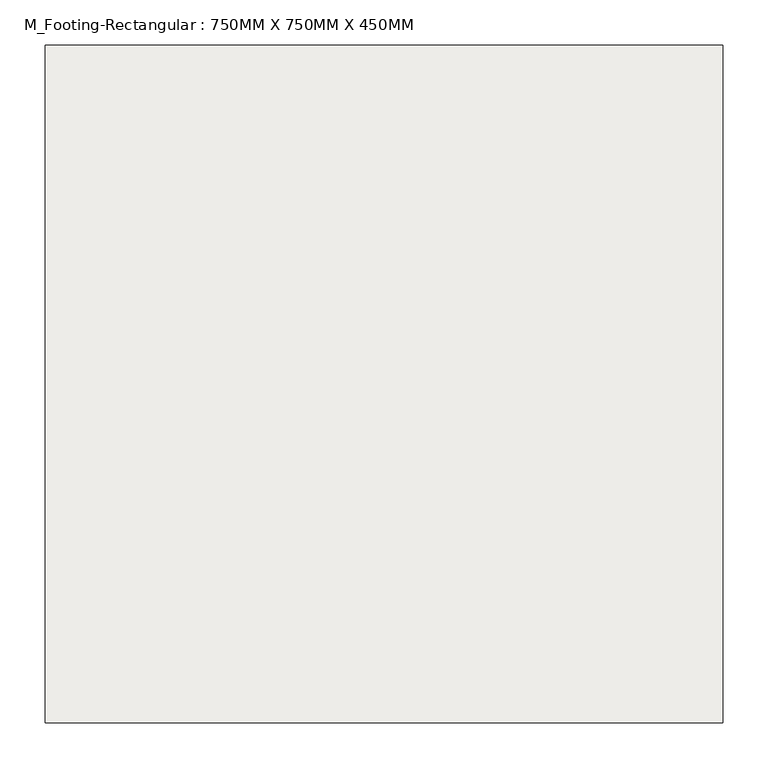
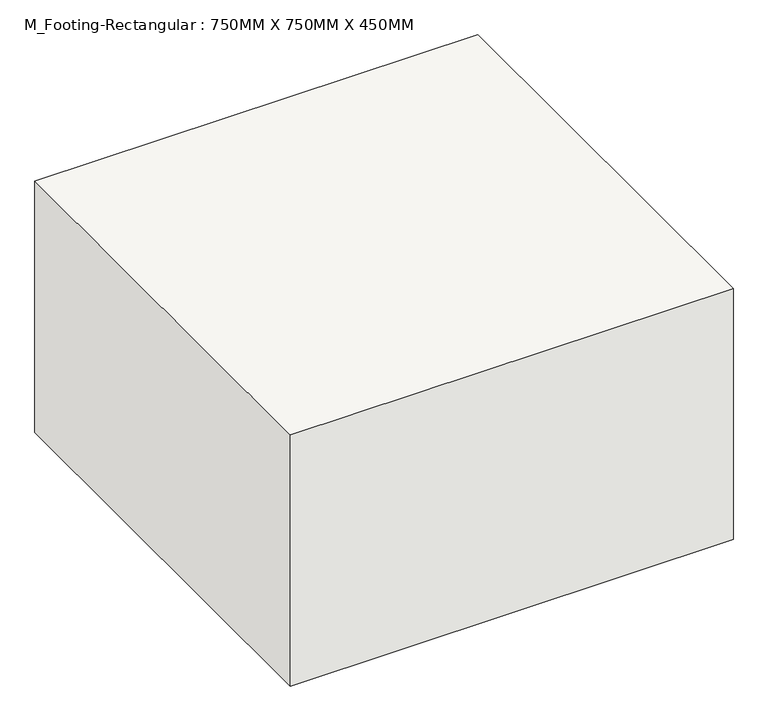
"""IFC4 building model written with IfcOpenShell, lengths in millimetres: slab geometry, M_Footing-Rectangular : 750MM X 750MM X 450MM."""

from ifc_helpers import new_model, si_unit, frame, origin, place, context, project, spatial, polyline, outline, extrude, source, transform, mapped, element, save


def m_footing_rectangular_750mm_x_750mm_x_450mm_d1bf6791(model_context):
    return source(origin(), model_context, "Body", "SweptSolid", [
        extrude(outline(polyline([(375.0, 375.0), (375.0, -375.0), (-375.0, -375.0), (-375.0, 375.0), (375.0, 375.0)])), frame((0.0, 0.0, -450.0), z_axis=(0.0, 0.0, 1.0), x_axis=(1.0, 0.0, 0.0)), (0.0, 0.0, 1.0), 450.0),
    ])


if __name__ == "__main__":
    model = new_model("IFC4")
    model_context = context("Model", 3, world=origin())
    ifc_project = project(units=[si_unit("LENGTHUNIT", "METRE", prefix="MILLI")], contexts=[model_context])
    site = spatial("IfcSite", under=ifc_project)
    building = spatial("IfcBuilding", under=site)
    placement = place(None, origin())
    m_footing_rectangular_750mm_x_750mm_x_450mm_shape = m_footing_rectangular_750mm_x_750mm_x_450mm_d1bf6791(model_context)
    element("IfcSlab", 1, ObjectType="M_Footing-Rectangular : 750MM X 750MM X 450MM", at=placement, inside=building, context=model_context, shape_type="MappedRepresentation", body=[
        mapped(m_footing_rectangular_750mm_x_750mm_x_450mm_shape, transform((0.0, 0.0, 0.0), x_axis=(1.0, 0.0, 0.0), y_axis=(0.0, 1.0, 0.0), z_axis=(0.0, 0.0, 1.0))),
    ])
    save(model, "model.ifc")

# Revit data of these elements
# Type "M_Footing-Rectangular : 750MM X 750MM X 450MM"
#   Width = 750 mm
#   Length = 750 mm
#   Foundation Thickness = 450 mm
#   Structural Material [instance default] = Concrete, Cast-in-Place gray
#   Assembly Code = ""
# Element 1 (IfcSlab, "M_Footing-Rectangular : 750MM X 750MM X 450MM")
#   Materials on its faces: "Concrete, Cast-in-Place gray"
# Materials
#   "Concrete, Cast-in-Place gray": class "Concrete", colour RGB 192 192 192, transparency 0, Description = "Cast-in-place concrete", Cost = 0
